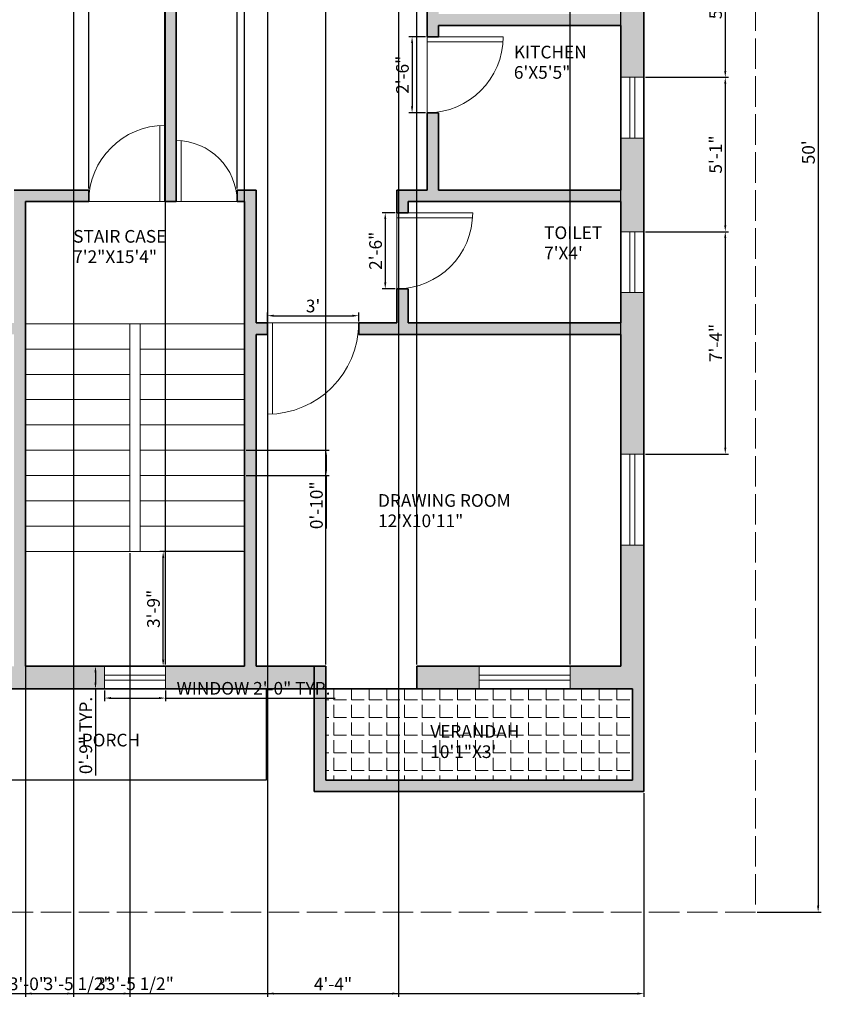
# Model space of a CAD drawing. Units: inches. Extents: x 2871 to 3419, y 1549 to 2228.
# Tile 2 of 3: x 3103 to 3419, y 1549 to 1938. Entities that reach past the tile are written whole.
import ezdxf

# ---------------------------------------------------------------- set-up
doc = ezdxf.new("R2010")
doc.units = ezdxf.units.IN
doc.linetypes.add('ACAD_ISO02W100', pattern=[15, 12, -3])
for name, color, linetype, lineweight in [('A-ANNO-DIMS', 3, 'Continuous', 13), ('A-AREA-IDEN', 3, 'Continuous', 18), ('A-FLOR', 7, 'Continuous', 25), ('A-FLOR-PATT', 30, 'Continuous', 13), ('A-FLOR-STRS', 61, 'Continuous', 18), ('A-WALL-PATT', 18, 'Continuous', 13), ('C-PROP', 7, 'ACAD_ISO02W100', 18), ('doors', 6, 'Continuous', 18), ('wall', 4, 'Continuous', 35), ('windows', 1, 'Continuous', 18)]:
    doc.layers.add(name, color=color, linetype=linetype, lineweight=lineweight)
doc.styles.get("Standard").update_dxf_attribs({"font": 'arial.ttf', "height": 5})
doc.dimstyles.new('ISO-25', dxfattribs={"dimtxt": 5, "dimasz": 2.5, "dimexe": 1.25, "dimexo": 0.625, "dimtad": 1, "dimlunit": 3, "dimtxsty": 'Standard', "dimcen": 2.5, "dimadec": 0, "dimazin": 0, "dimtfac": 1, "dimtmove": 0, "dimatfit": 3, "dimfxl": 1, "dimarcsym": 0})

# ---------------------------------------------------------------- blocks, each defined once
blk = doc.blocks.new('*D6')
at = {"layer": 'A-ANNO-DIMS', "color": 0, "lineweight": -2, "transparency": 16777216}
for p, q in [((3263.29, 1931.24), (3256.74, 1931.24)), ((3257.99, 1928.74), (3257.99, 1903.74)), ((3263.29, 1901.24), (3256.74, 1901.24))]:
    blk.add_line(p, q, dxfattribs=at)
at = {"layer": 'A-ANNO-DIMS', "color": 0, "transparency": 16777216}
for points in [[(3257.58, 1928.74), (3258.41, 1928.74), (3257.99, 1931.24)], [(3257.58, 1903.74), (3258.41, 1903.74), (3257.99, 1901.24)]]:
    blk.add_solid(points, dxfattribs=at)
at = {"layer": 'Defpoints', "color": 0, "transparency": 16777216}
for p in [(3263.92, 1931.24), (3257.99, 1901.24), (3263.92, 1901.24)]:
    blk.add_point(p, dxfattribs=at)
at = {"layer": 'A-ANNO-DIMS', "color": 0, "transparency": 16777216, "insert": (3254.82, 1916.24), "char_height": 5, "attachment_point": 5, "rotation": 90}
blk.add_mtext('2\'-6"', dxfattribs=at)
blk = doc.blocks.new('*D7')
at = {"layer": 'A-ANNO-DIMS', "color": 0, "lineweight": -2, "transparency": 16777216}
for p, q in [((3251.29, 1861.74), (3246.15, 1861.74)), ((3247.4, 1859.24), (3247.4, 1834.24)), ((3251.29, 1831.74), (3246.15, 1831.74))]:
    blk.add_line(p, q, dxfattribs=at)
at = {"layer": 'A-ANNO-DIMS', "color": 0, "transparency": 16777216}
for points in [[(3246.99, 1859.24), (3247.82, 1859.24), (3247.4, 1861.74)], [(3246.99, 1834.24), (3247.82, 1834.24), (3247.4, 1831.74)]]:
    blk.add_solid(points, dxfattribs=at)
at = {"layer": 'Defpoints', "color": 0, "transparency": 16777216}
for p in [(3251.92, 1861.74), (3247.4, 1831.74), (3251.92, 1831.74)]:
    blk.add_point(p, dxfattribs=at)
at = {"layer": 'A-ANNO-DIMS', "color": 0, "transparency": 16777216, "insert": (3244.23, 1846.74), "char_height": 5, "attachment_point": 5, "rotation": 90}
blk.add_mtext('2\'-6"', dxfattribs=at)
blk = doc.blocks.new('*D8')
at = {"layer": 'A-ANNO-DIMS', "color": 0, "lineweight": -2, "transparency": 16777216}
for p, q in [((3200.92, 1818.86), (3200.92, 1822.36)), ((3203.42, 1821.11), (3234.42, 1821.11)), ((3236.92, 1818.86), (3236.92, 1822.36))]:
    blk.add_line(p, q, dxfattribs=at)
at = {"layer": 'A-ANNO-DIMS', "color": 0, "transparency": 16777216}
for points in [[(3203.42, 1821.53), (3203.42, 1820.69), (3200.92, 1821.11)], [(3234.42, 1821.53), (3234.42, 1820.69), (3236.92, 1821.11)]]:
    blk.add_solid(points, dxfattribs=at)
at = {"layer": 'Defpoints', "color": 0, "transparency": 16777216}
for p in [(3236.92, 1821.11), (3200.92, 1818.24), (3236.92, 1818.24)]:
    blk.add_point(p, dxfattribs=at)
at = {"layer": 'A-ANNO-DIMS', "color": 0, "transparency": 16777216, "insert": (3218.92, 1824.29), "char_height": 5, "attachment_point": 5}
blk.add_mtext("3'", dxfattribs=at)
blk = doc.blocks.new('*D13')
at = {"layer": 'A-ANNO-DIMS', "color": 0, "lineweight": -2, "transparency": 16777216}
for p, q in [((3394.09, 2185.62), (3419.45, 2185.62)), ((3418.2, 2183.12), (3418.2, 1588.12)), ((3394.09, 1585.62), (3419.45, 1585.62))]:
    blk.add_line(p, q, dxfattribs=at)
at = {"layer": 'A-ANNO-DIMS', "color": 0, "transparency": 16777216}
for points in [[(3417.79, 2183.12), (3418.62, 2183.12), (3418.2, 2185.62)], [(3417.79, 1588.12), (3418.62, 1588.12), (3418.2, 1585.62)]]:
    blk.add_solid(points, dxfattribs=at)
at = {"layer": 'Defpoints', "color": 0, "transparency": 16777216}
for p in [(3393.47, 2185.62), (3393.47, 1585.62), (3418.2, 1585.62)]:
    blk.add_point(p, dxfattribs=at)
at = {"layer": 'A-ANNO-DIMS', "color": 0, "transparency": 16777216, "insert": (3415.03, 1885.62), "char_height": 5, "attachment_point": 5, "rotation": 90}
blk.add_mtext("50'", dxfattribs=at)
blk = doc.blocks.new('WIN-36IN')
for p, q in [((0, 36), (0, 0)), ((9, 36), (0, 36)), ((3.5, 0), (3.5, 36)), ((5.5, 0), (5.5, 36)), ((9, 0), (9, 36)), ((0, 0), (9, 0))]:
    blk.add_line(p, q)
blk = doc.blocks.new('WIN-24IN')
for p, q in [((0, 24), (0, 0)), ((9, 24), (0, 24)), ((3.5, 0), (3.5, 24)), ((5.5, 0), (5.5, 24)), ((9, 0), (9, 24)), ((0, 0), (9, 0))]:
    blk.add_line(p, q)
blk = doc.blocks.new('DOOR-SWING-30IN')
for p, q in [((28, 29.93), (28, 0)), ((30, 30), (30, 0)), ((30, 0), (0, 0))]:
    blk.add_line(p, q)
blk.add_arc((30, 0), 30, 90, 180)
blk = doc.blocks.new('DOOR-SWING-36IN')
for p, q in [((0, 36), (0, 0)), ((2, 35.94), (2, 0)), ((0, 0), (36, 0))]:
    blk.add_line(p, q)
blk.add_arc((0, 0), 36, 0, 90)
blk = doc.blocks.new('*D20')
at = {"layer": 'A-ANNO-DIMS', "color": 0, "lineweight": -2, "transparency": 16777216}
for p, q in [((3136.67, 1673.11), (3136.67, 1668.89)), ((3160.67, 1673.11), (3160.67, 1668.89)), ((3139.17, 1670.14), (3158.17, 1670.14)), ((3160.67, 1670.14), (3227.69, 1670.14))]:
    blk.add_line(p, q, dxfattribs=at)
at = {"layer": 'A-ANNO-DIMS', "color": 0, "transparency": 16777216}
for points in [[(3139.17, 1670.55), (3139.17, 1669.72), (3136.67, 1670.14)], [(3158.17, 1670.55), (3158.17, 1669.72), (3160.67, 1670.14)]]:
    blk.add_solid(points, dxfattribs=at)
at = {"layer": 'Defpoints', "color": 0, "transparency": 16777216}
for p in [(3136.67, 1673.74), (3160.67, 1673.74), (3160.67, 1670.14)]:
    blk.add_point(p, dxfattribs=at)
at = {"layer": 'A-ANNO-DIMS', "color": 0, "transparency": 16777216, "insert": (3195.43, 1673.35), "char_height": 5, "attachment_point": 5}
blk.add_mtext('WINDOW 2\'-0" TYP.', dxfattribs=at)
blk = doc.blocks.new('*D21')
at = {"layer": 'A-ANNO-DIMS', "color": 0, "lineweight": -2, "transparency": 16777216}
for p, q in [((3136.04, 1682.74), (3131.82, 1682.74)), ((3133.07, 1680.24), (3133.07, 1676.24)), ((3136.04, 1673.74), (3131.82, 1673.74)), ((3133.07, 1673.74), (3133.07, 1639.51))]:
    blk.add_line(p, q, dxfattribs=at)
at = {"layer": 'A-ANNO-DIMS', "color": 0, "transparency": 16777216}
for points in [[(3132.65, 1680.24), (3133.48, 1680.24), (3133.07, 1682.74)], [(3132.65, 1676.24), (3133.48, 1676.24), (3133.07, 1673.74)]]:
    blk.add_solid(points, dxfattribs=at)
at = {"layer": 'Defpoints', "color": 0, "transparency": 16777216}
for p in [(3136.67, 1682.74), (3133.07, 1673.74), (3136.67, 1673.74)]:
    blk.add_point(p, dxfattribs=at)
at = {"layer": 'A-ANNO-DIMS', "color": 0, "transparency": 16777216, "insert": (3129.89, 1655.37), "char_height": 5, "attachment_point": 5, "rotation": 90}
blk.add_mtext('0\'-9" TYP.', dxfattribs=at)
blk = doc.blocks.new('*D22')
at = {"layer": 'A-ANNO-DIMS', "color": 0, "lineweight": -2, "transparency": 16777216}
for p, q in [((2947.92, 1632.61), (2947.92, 1552.22)), ((3349.42, 1632.61), (3349.42, 1552.22)), ((2950.42, 1553.47), (3346.92, 1553.47))]:
    blk.add_line(p, q, dxfattribs=at)
at = {"layer": 'A-ANNO-DIMS', "color": 0, "transparency": 16777216}
for points in [[(2950.42, 1553.89), (2950.42, 1553.05), (2947.92, 1553.47)], [(3346.92, 1553.89), (3346.92, 1553.05), (3349.42, 1553.47)]]:
    blk.add_solid(points, dxfattribs=at)
at = {"layer": 'Defpoints', "color": 0, "transparency": 16777216}
for p in [(2947.92, 1633.24), (3349.42, 1633.24), (3349.42, 1553.47)]:
    blk.add_point(p, dxfattribs=at)
at = {"layer": 'A-ANNO-DIMS', "color": 0, "transparency": 16777216, "insert": (3148.67, 1556.68), "char_height": 5, "attachment_point": 5}
blk.add_mtext('33\'-5 1/2"', dxfattribs=at)
blk = doc.blocks.new('*D27')
at = {"layer": 'A-ANNO-DIMS', "color": 0, "lineweight": -2, "transparency": 16777216}
for p, q in [((3088.42, 2131.11), (3088.42, 1552.22)), ((3124.42, 2131.11), (3124.42, 1552.22)), ((3090.92, 1553.47), (3121.92, 1553.47))]:
    blk.add_line(p, q, dxfattribs=at)
at = {"layer": 'A-ANNO-DIMS', "color": 0, "transparency": 16777216}
for points in [[(3090.92, 1553.89), (3090.92, 1553.05), (3088.42, 1553.47)], [(3121.92, 1553.89), (3121.92, 1553.05), (3124.42, 1553.47)]]:
    blk.add_solid(points, dxfattribs=at)
at = {"layer": 'Defpoints', "color": 0, "transparency": 16777216}
for p in [(3088.42, 2131.74), (3124.42, 2131.74), (3124.42, 1553.47)]:
    blk.add_point(p, dxfattribs=at)
at = {"layer": 'A-ANNO-DIMS', "color": 0, "transparency": 16777216, "insert": (3106.42, 1556.65), "char_height": 5, "attachment_point": 5}
blk.add_mtext('3\'-0"', dxfattribs=at)
blk = doc.blocks.new('*D28')
at = {"layer": 'A-ANNO-DIMS', "color": 0, "lineweight": -2, "transparency": 16777216}
for p, q in [((3200.92, 2131.11), (3200.92, 1552.22)), ((3252.67, 2131.11), (3252.67, 1552.22)), ((3203.42, 1553.47), (3250.17, 1553.47))]:
    blk.add_line(p, q, dxfattribs=at)
at = {"layer": 'A-ANNO-DIMS', "color": 0, "transparency": 16777216}
for points in [[(3203.42, 1553.89), (3203.42, 1553.05), (3200.92, 1553.47)], [(3250.17, 1553.89), (3250.17, 1553.05), (3252.67, 1553.47)]]:
    blk.add_solid(points, dxfattribs=at)
at = {"layer": 'Defpoints', "color": 0, "transparency": 16777216}
for p in [(3200.92, 2131.74), (3252.67, 2131.74), (3252.67, 1553.47)]:
    blk.add_point(p, dxfattribs=at)
at = {"layer": 'A-ANNO-DIMS', "color": 0, "transparency": 16777216, "insert": (3226.79, 1556.6), "char_height": 5, "attachment_point": 5}
blk.add_mtext('4\'-4"', dxfattribs=at)
blk = doc.blocks.new('*D29')
at = {"layer": 'A-ANNO-DIMS', "color": 0, "lineweight": -2, "transparency": 16777216}
for p, q in [((3130.42, 1871.36), (3130.42, 2219.02)), ((3132.92, 2217.77), (3157.92, 2217.77)), ((3160.42, 1871.36), (3160.42, 2219.02))]:
    blk.add_line(p, q, dxfattribs=at)
at = {"layer": 'A-ANNO-DIMS', "color": 0, "transparency": 16777216}
for points in [[(3132.92, 2218.19), (3132.92, 2217.35), (3130.42, 2217.77)], [(3157.92, 2218.19), (3157.92, 2217.35), (3160.42, 2217.77)]]:
    blk.add_solid(points, dxfattribs=at)
at = {"layer": 'Defpoints', "color": 0, "transparency": 16777216}
for p in [(3160.42, 2217.77), (3130.42, 1870.74), (3160.42, 1870.74)]:
    blk.add_point(p, dxfattribs=at)
at = {"layer": 'A-ANNO-DIMS', "color": 0, "transparency": 16777216, "insert": (3145.42, 2220.95), "char_height": 5, "attachment_point": 5}
blk.add_mtext('2\'-6"', dxfattribs=at)
blk = doc.blocks.new('*D30')
at = {"layer": 'A-ANNO-DIMS', "color": 0, "lineweight": -2, "transparency": 16777216}
for p, q in [((3164.92, 1871.36), (3164.92, 2219.02)), ((3167.42, 2217.77), (3186.42, 2217.77)), ((3188.92, 1871.36), (3188.92, 2219.02))]:
    blk.add_line(p, q, dxfattribs=at)
at = {"layer": 'A-ANNO-DIMS', "color": 0, "transparency": 16777216}
for points in [[(3167.42, 2218.19), (3167.42, 2217.35), (3164.92, 2217.77)], [(3186.42, 2218.19), (3186.42, 2217.35), (3188.92, 2217.77)]]:
    blk.add_solid(points, dxfattribs=at)
at = {"layer": 'Defpoints', "color": 0, "transparency": 16777216}
for p in [(3188.92, 2217.77), (3164.92, 1870.74), (3188.92, 1870.74)]:
    blk.add_point(p, dxfattribs=at)
at = {"layer": 'A-ANNO-DIMS', "color": 0, "transparency": 16777216, "insert": (3176.92, 2220.95), "char_height": 5, "attachment_point": 5}
blk.add_mtext('2\'-0"', dxfattribs=at)
blk = doc.blocks.new('*D31')
at = {"layer": 'A-ANNO-DIMS', "color": 0, "lineweight": -2, "transparency": 16777216}
for p, q in [((3191.29, 1727.96), (3158.52, 1727.96)), ((3159.77, 1685.24), (3159.77, 1725.46)), ((3191.29, 1682.74), (3158.52, 1682.74))]:
    blk.add_line(p, q, dxfattribs=at)
at = {"layer": 'A-ANNO-DIMS', "color": 0, "transparency": 16777216}
for points in [[(3159.35, 1725.46), (3160.18, 1725.46), (3159.77, 1727.96)], [(3159.35, 1685.24), (3160.18, 1685.24), (3159.77, 1682.74)]]:
    blk.add_solid(points, dxfattribs=at)
at = {"layer": 'Defpoints', "color": 0, "transparency": 16777216}
for p in [(3159.77, 1727.96), (3191.92, 1727.96), (3191.92, 1682.74)]:
    blk.add_point(p, dxfattribs=at)
at = {"layer": 'A-ANNO-DIMS', "color": 0, "transparency": 16777216, "insert": (3156.59, 1705.35), "char_height": 5, "attachment_point": 5, "rotation": 90}
blk.add_mtext('3\'-9"', dxfattribs=at)
blk = doc.blocks.new('*D32')
at = {"layer": 'A-ANNO-DIMS', "color": 0, "lineweight": -2, "transparency": 16777216}
for p, q in [((3192.54, 1767.96), (3225.32, 1767.96)), ((3224.07, 1765.46), (3224.07, 1760.46)), ((3192.54, 1757.96), (3225.32, 1757.96)), ((3224.07, 1757.96), (3224.07, 1737.03))]:
    blk.add_line(p, q, dxfattribs=at)
at = {"layer": 'A-ANNO-DIMS', "color": 0, "transparency": 16777216}
for points in [[(3223.65, 1765.46), (3224.48, 1765.46), (3224.07, 1767.96)], [(3223.65, 1760.46), (3224.48, 1760.46), (3224.07, 1757.96)]]:
    blk.add_solid(points, dxfattribs=at)
at = {"layer": 'Defpoints', "color": 0, "transparency": 16777216}
for p in [(3191.92, 1767.96), (3191.92, 1757.96), (3224.07, 1757.96)]:
    blk.add_point(p, dxfattribs=at)
at = {"layer": 'A-ANNO-DIMS', "color": 0, "transparency": 16777216, "insert": (3220.89, 1746.25), "char_height": 5, "attachment_point": 5, "rotation": 90}
blk.add_mtext('0\'-10"', dxfattribs=at)
blk = doc.blocks.new('*D33')
at = {"layer": 'A-ANNO-DIMS', "color": 0, "lineweight": -2, "transparency": 16777216}
for p, q in [((3105.42, 1727.34), (3105.42, 1552.22)), ((3146.67, 1727.34), (3146.67, 1552.22)), ((3107.92, 1553.47), (3144.17, 1553.47))]:
    blk.add_line(p, q, dxfattribs=at)
at = {"layer": 'A-ANNO-DIMS', "color": 0, "transparency": 16777216}
for points in [[(3107.92, 1553.89), (3107.92, 1553.05), (3105.42, 1553.47)], [(3144.17, 1553.89), (3144.17, 1553.05), (3146.67, 1553.47)]]:
    blk.add_solid(points, dxfattribs=at)
at = {"layer": 'Defpoints', "color": 0, "transparency": 16777216}
for p in [(3105.42, 1727.96), (3146.67, 1727.96), (3146.67, 1553.47)]:
    blk.add_point(p, dxfattribs=at)
at = {"layer": 'A-ANNO-DIMS', "color": 0, "transparency": 16777216, "insert": (3126.04, 1556.68), "char_height": 5, "attachment_point": 5}
blk.add_mtext('3\'-5 1/2"', dxfattribs=at)
blk = doc.blocks.new('*D36')
at = {"layer": 'A-ANNO-DIMS', "color": 0, "lineweight": -2, "transparency": 16777216}
for p, q in [((3350.04, 1976.24), (3382.82, 1976.24)), ((3381.57, 1973.74), (3381.57, 1917.74)), ((3350.04, 1915.24), (3382.82, 1915.24))]:
    blk.add_line(p, q, dxfattribs=at)
at = {"layer": 'A-ANNO-DIMS', "color": 0, "transparency": 16777216}
for points in [[(3381.15, 1973.74), (3381.98, 1973.74), (3381.57, 1976.24)], [(3381.15, 1917.74), (3381.98, 1917.74), (3381.57, 1915.24)]]:
    blk.add_solid(points, dxfattribs=at)
at = {"layer": 'Defpoints', "color": 0, "transparency": 16777216}
for p in [(3349.42, 1976.24), (3349.42, 1915.24), (3381.57, 1915.24)]:
    blk.add_point(p, dxfattribs=at)
at = {"layer": 'A-ANNO-DIMS', "color": 0, "transparency": 16777216, "insert": (3378.39, 1945.74), "char_height": 5, "attachment_point": 5, "rotation": 90}
blk.add_mtext('5\'-1"', dxfattribs=at)
blk = doc.blocks.new('*D37')
at = {"layer": 'A-ANNO-DIMS', "color": 0, "lineweight": -2, "transparency": 16777216}
for p, q in [((3350.04, 1915.24), (3382.82, 1915.24)), ((3381.57, 1912.74), (3381.57, 1856.74)), ((3350.04, 1854.24), (3382.82, 1854.24))]:
    blk.add_line(p, q, dxfattribs=at)
at = {"layer": 'A-ANNO-DIMS', "color": 0, "transparency": 16777216}
for points in [[(3381.15, 1912.74), (3381.98, 1912.74), (3381.57, 1915.24)], [(3381.15, 1856.74), (3381.98, 1856.74), (3381.57, 1854.24)]]:
    blk.add_solid(points, dxfattribs=at)
at = {"layer": 'Defpoints', "color": 0, "transparency": 16777216}
for p in [(3349.42, 1915.24), (3349.42, 1854.24), (3381.57, 1854.24)]:
    blk.add_point(p, dxfattribs=at)
at = {"layer": 'A-ANNO-DIMS', "color": 0, "transparency": 16777216, "insert": (3378.39, 1884.74), "char_height": 5, "attachment_point": 5, "rotation": 90}
blk.add_mtext('5\'-1"', dxfattribs=at)
blk = doc.blocks.new('*D38')
at = {"layer": 'A-ANNO-DIMS', "color": 0, "lineweight": -2, "transparency": 16777216}
for p, q in [((3350.04, 1854.24), (3382.82, 1854.24)), ((3381.57, 1851.74), (3381.57, 1768.95)), ((3350.04, 1766.45), (3382.82, 1766.45))]:
    blk.add_line(p, q, dxfattribs=at)
at = {"layer": 'A-ANNO-DIMS', "color": 0, "transparency": 16777216}
for points in [[(3381.15, 1851.74), (3381.98, 1851.74), (3381.57, 1854.24)], [(3381.15, 1768.95), (3381.98, 1768.95), (3381.57, 1766.45)]]:
    blk.add_solid(points, dxfattribs=at)
at = {"layer": 'Defpoints', "color": 0, "transparency": 16777216}
for p in [(3349.42, 1854.24), (3349.42, 1766.45), (3381.57, 1766.45)]:
    blk.add_point(p, dxfattribs=at)
at = {"layer": 'A-ANNO-DIMS', "color": 0, "transparency": 16777216, "insert": (3378.44, 1810.34), "char_height": 5, "attachment_point": 5, "rotation": 90}
blk.add_mtext('7\'-4"', dxfattribs=at)
blk = doc.blocks.new('*D45')
at = {"layer": 'A-ANNO-DIMS', "color": 0, "lineweight": -2, "transparency": 16777216}
for p, q in [((3320.42, 1683.36), (3320.42, 2219.02)), ((3322.92, 2217.77), (3337.92, 2217.77)), ((3340.42, 1683.36), (3340.42, 2219.02))]:
    blk.add_line(p, q, dxfattribs=at)
at = {"layer": 'A-ANNO-DIMS', "color": 0, "transparency": 16777216}
for points in [[(3322.92, 2218.19), (3322.92, 2217.35), (3320.42, 2217.77)], [(3337.92, 2218.19), (3337.92, 2217.35), (3340.42, 2217.77)]]:
    blk.add_solid(points, dxfattribs=at)
at = {"layer": 'Defpoints', "color": 0, "transparency": 16777216}
for p in [(3340.42, 2217.77), (3320.42, 1682.74), (3340.42, 1682.74)]:
    blk.add_point(p, dxfattribs=at)
at = {"layer": 'A-ANNO-DIMS', "color": 0, "transparency": 16777216, "insert": (3330.42, 2220.95), "char_height": 5, "attachment_point": 5}
blk.add_mtext('1\'-8"', dxfattribs=at)
blk = doc.blocks.new('*D47')
at = {"layer": 'A-ANNO-DIMS', "color": 0, "lineweight": -2, "transparency": 16777216}
for p, q in [((3223.92, 1683.36), (3223.92, 2219.02)), ((3226.42, 2217.77), (3257.42, 2217.77)), ((3259.92, 1683.36), (3259.92, 2219.02))]:
    blk.add_line(p, q, dxfattribs=at)
at = {"layer": 'A-ANNO-DIMS', "color": 0, "transparency": 16777216}
for points in [[(3226.42, 2218.19), (3226.42, 2217.35), (3223.92, 2217.77)], [(3257.42, 2218.19), (3257.42, 2217.35), (3259.92, 2217.77)]]:
    blk.add_solid(points, dxfattribs=at)
at = {"layer": 'Defpoints', "color": 0, "transparency": 16777216}
for p in [(3259.92, 2217.77), (3223.92, 1682.74), (3259.92, 1682.74)]:
    blk.add_point(p, dxfattribs=at)
at = {"layer": 'A-ANNO-DIMS', "color": 0, "transparency": 16777216, "insert": (3241.92, 2220.95), "char_height": 5, "attachment_point": 5}
blk.add_mtext('3\'-0"', dxfattribs=at)
blk = doc.blocks.new('*D49')
at = {"layer": 'A-ANNO-DIMS', "color": 0, "lineweight": -2, "transparency": 16777216}
for p, q in [((3259.92, 1683.36), (3259.92, 2219.02)), ((3262.42, 2217.77), (3317.92, 2217.77)), ((3320.42, 1683.36), (3320.42, 2219.02))]:
    blk.add_line(p, q, dxfattribs=at)
at = {"layer": 'A-ANNO-DIMS', "color": 0, "transparency": 16777216}
for points in [[(3262.42, 2218.19), (3262.42, 2217.35), (3259.92, 2217.77)], [(3317.92, 2218.19), (3317.92, 2217.35), (3320.42, 2217.77)]]:
    blk.add_solid(points, dxfattribs=at)
at = {"layer": 'Defpoints', "color": 0, "transparency": 16777216}
for p in [(3320.42, 2217.77), (3259.92, 1682.74), (3320.42, 1682.74)]:
    blk.add_point(p, dxfattribs=at)
at = {"layer": 'A-ANNO-DIMS', "color": 0, "transparency": 16777216, "insert": (3290.17, 2220.98), "char_height": 5, "attachment_point": 5}
blk.add_mtext('5\'-0 1/2"', dxfattribs=at)
blk = doc.blocks.new('*D51')
at = {"layer": 'A-ANNO-DIMS', "color": 0, "lineweight": -2, "transparency": 16777216}
for p, q in [((3160.67, 1683.36), (3160.67, 2219.02)), ((3163.17, 2217.77), (3189.42, 2217.77)), ((3191.92, 1683.36), (3191.92, 2219.02))]:
    blk.add_line(p, q, dxfattribs=at)
at = {"layer": 'A-ANNO-DIMS', "color": 0, "transparency": 16777216}
for points in [[(3163.17, 2218.19), (3163.17, 2217.35), (3160.67, 2217.77)], [(3189.42, 2218.19), (3189.42, 2217.35), (3191.92, 2217.77)]]:
    blk.add_solid(points, dxfattribs=at)
at = {"layer": 'Defpoints', "color": 0, "transparency": 16777216}
for p in [(3191.92, 2217.77), (3160.67, 1682.74), (3191.92, 1682.74)]:
    blk.add_point(p, dxfattribs=at)
at = {"layer": 'A-ANNO-DIMS', "color": 0, "transparency": 16777216, "insert": (3176.29, 2220.98), "char_height": 5, "attachment_point": 5}
blk.add_mtext('2\'-7 1/2"', dxfattribs=at)

msp = doc.modelspace()

# ---------------------------------------------------------------- hatches: boundary and pattern name
at = {"layer": 'A-FLOR-PATT'}
h = msp.add_hatch(dxfattribs=at)
h.set_pattern_fill('ANGLE', color=256)
h.set_pattern_definition([(0, (0, 0), (0, 6.985), [5.08, -1.905]), (90, (0, 0), (-6.985, 4e-16), [5.08, -1.905])])
h.paths.add_polyline_path([(3073.418, 1673.735), (3037.418, 1673.735), (2952.418, 1673.735), (2952.418, 1637.735), (3073.418, 1637.735)])
h.paths.add_polyline_path([(3344.918, 1673.735), (3259.918, 1673.735), (3223.918, 1673.735), (3223.918, 1637.735), (3344.918, 1637.735)])
h.paths.add_polyline_path([(2998.155, 1645.095), (3026.055, 1645.095), (3026.055, 1652.758), (2998.155, 1652.758)], flags=24)
h.paths.add_polyline_path([(2998.183, 1653.243), (3039.496, 1653.243), (3039.496, 1660.743), (2998.183, 1660.743)], flags=24)
h.paths.add_polyline_path([(3263.884, 1645.095), (3291.783, 1645.095), (3291.783, 1652.758), (3263.884, 1652.758)], flags=24)
h.paths.add_polyline_path([(3263.911, 1653.243), (3305.224, 1653.243), (3305.224, 1660.743), (3263.911, 1660.743)], flags=24)
at = {"layer": 'A-WALL-PATT'}
h = msp.add_hatch(color=256, dxfattribs=at)
h.dxf.hatch_style = 1
h.paths.add_polyline_path([(2956.918, 2131.735), (3002.418, 2131.735), (3002.418, 2140.735), (2947.918, 2140.735), (2947.918, 2079.154), (2956.918, 2079.154)])
h.paths.add_polyline_path([(3252.668, 2140.735), (3160.418, 2140.735), (3160.418, 2131.735), (3196.418, 2131.735), (3196.418, 1992.735), (3128.918, 1992.735), (3128.918, 1988.235), (3160.418, 1988.235), (3160.418, 1870.735), (3160.418, 1866.235), (3164.918, 1866.235), (3164.918, 1890.235), (3164.918, 1988.235), (3205.418, 1988.235), (3205.418, 1992.735), (3200.918, 1992.735), (3200.918, 2131.735), (3252.668, 2131.735)])
h.paths.add_polyline_path([(3349.418, 2140.735), (3288.668, 2140.735), (3288.668, 2131.735), (3340.418, 2131.735), (3340.418, 2080.235), (3349.418, 2080.235)])
h.paths.add_polyline_path([(3349.418, 2044.235), (3340.418, 2044.235), (3340.418, 1992.735), (3302.918, 1992.735), (3302.918, 1988.235), (3340.418, 1988.235), (3340.418, 1976.235), (3349.418, 1976.235)])
h.paths.add_polyline_path([(3349.418, 1952.235), (3340.418, 1952.235), (3340.418, 1940.235), (3268.418, 1940.235), (3268.418, 1988.235), (3272.918, 1988.235), (3272.918, 1992.735), (3241.418, 1992.735), (3241.418, 1988.235), (3263.918, 1988.235), (3263.918, 1931.235), (3268.418, 1931.235), (3268.418, 1935.735), (3340.418, 1935.735), (3340.418, 1915.235), (3349.418, 1915.235)])
h.paths.add_polyline_path([(3349.418, 1891.235), (3340.418, 1891.235), (3340.418, 1870.735), (3268.418, 1870.735), (3268.418, 1901.235), (3263.918, 1901.235), (3263.918, 1870.735), (3251.918, 1870.735), (3251.918, 1866.235), (3251.918, 1861.735), (3256.418, 1861.735), (3256.418, 1866.235), (3340.418, 1866.235), (3340.418, 1854.235), (3349.418, 1854.235)])
h.paths.add_polyline_path([(3349.418, 1830.235), (3340.418, 1830.235), (3340.418, 1818.235), (3256.418, 1818.235), (3256.418, 1831.735), (3251.918, 1831.735), (3251.918, 1818.235), (3236.918, 1818.235), (3236.918, 1813.735), (3340.418, 1813.735), (3340.418, 1766.452), (3349.418, 1766.452)])
h.paths.add_polyline_path([(3349.418, 1730.452), (3340.418, 1730.452), (3340.418, 1682.735), (3320.418, 1682.735), (3320.418, 1673.735), (3344.918, 1673.735), (3344.918, 1637.735), (3223.918, 1637.735), (3223.918, 1673.735), (3219.418, 1673.735), (3219.418, 1633.235), (3349.418, 1633.235)])
h.paths.add_polyline_path([(3284.418, 1682.735), (3259.918, 1682.735), (3259.918, 1673.735), (3284.418, 1673.735)], flags=17)
h.paths.add_polyline_path([(3223.918, 1682.735), (3219.418, 1682.735), (3219.418, 1673.735), (3223.918, 1673.735)], flags=17)
h.paths.add_polyline_path([(3196.418, 1813.735), (3200.918, 1813.735), (3200.918, 1818.235), (3196.418, 1818.235), (3196.418, 1866.235), (3196.418, 1870.735), (3188.918, 1870.735), (3188.918, 1866.235), (3191.918, 1866.235), (3191.918, 1682.735), (3160.668, 1682.735), (3160.668, 1673.735), (3219.418, 1673.735), (3219.418, 1682.735), (3196.418, 1682.735)])
h.paths.add_polyline_path([(3105.418, 1866.235), (3130.418, 1866.235), (3130.418, 1870.735), (3100.918, 1870.735), (3100.918, 1866.235), (3100.918, 1818.235), (3096.418, 1818.235), (3096.418, 1813.735), (3100.918, 1813.735), (3100.918, 1682.735), (3077.918, 1682.735), (3077.918, 1673.735), (3136.668, 1673.735), (3136.668, 1682.735), (3105.418, 1682.735)])
h.paths.add_polyline_path([(3077.918, 1682.735), (3073.418, 1682.735), (3073.418, 1673.735), (3077.918, 1673.735)], flags=17)
h.paths.add_polyline_path([(3077.918, 1673.735), (3073.418, 1673.735), (3073.418, 1637.735), (2952.418, 1637.735), (2952.418, 1673.735), (2976.918, 1673.735), (2976.918, 1682.735), (2956.918, 1682.735), (2956.918, 1729.593), (2947.918, 1729.593), (2947.918, 1633.235), (3077.918, 1633.235)])
h.paths.add_polyline_path([(3037.418, 1682.735), (3012.918, 1682.735), (3012.918, 1673.735), (3037.418, 1673.735)], flags=17)
h.paths.add_polyline_path([(3060.418, 1818.235), (3045.418, 1818.235), (3045.418, 1831.735), (3040.918, 1831.735), (3040.918, 1818.235), (2956.918, 1818.235), (2956.918, 1830.772), (2947.918, 1830.772), (2947.918, 1765.593), (2956.918, 1765.593), (2956.918, 1813.735), (3060.418, 1813.735)])
h.paths.add_polyline_path([(3045.418, 1870.735), (3033.418, 1870.735), (3033.418, 1901.235), (3028.918, 1901.235), (3028.918, 1870.735), (2956.918, 1870.735), (2956.918, 1891.289), (2947.918, 1891.289), (2947.918, 1854.772), (2956.918, 1854.772), (2956.918, 1866.235), (3040.918, 1866.235), (3040.918, 1861.735), (3045.418, 1861.735), (3045.418, 1866.235)])
h.paths.add_polyline_path([(3033.418, 1988.235), (3043.418, 1988.235), (3043.418, 1992.735), (3024.418, 1992.735), (3024.418, 1988.235), (3028.918, 1988.235), (3028.918, 1940.235), (2956.918, 1940.235), (2956.918, 1952.063), (2947.918, 1952.063), (2947.918, 1915.289), (2956.918, 1915.289), (2956.918, 1935.735), (3028.918, 1935.735), (3028.918, 1931.235), (3033.418, 1931.235)])
h.paths.add_polyline_path([(2956.918, 2043.154), (2947.918, 2043.154), (2947.918, 1976.063), (2956.918, 1976.063), (2956.918, 1988.235), (2994.418, 1988.235), (2994.418, 1992.735), (2956.918, 1992.735)])

# ---------------------------------------------------------------- linework, layer by layer
at = {"layer": 'A-FLOR'}
for p, q in [((3200.352, 1673.735), (3200.352, 1637.735)), ((3200.352, 1637.735), (3097.318, 1637.735))]:
    msp.add_line(p, q, dxfattribs=at)
at = {"layer": 'A-FLOR-STRS'}
for p, q in [((3191.918, 1817.96), (3105.418, 1817.96)), ((3146.668, 1817.96), (3146.668, 1727.96)), ((3150.668, 1817.96), (3150.668, 1727.96)), ((3146.668, 1807.96), (3105.418, 1807.96)), ((3191.918, 1807.96), (3150.668, 1807.96)), ((3146.668, 1797.96), (3105.418, 1797.96)), ((3191.918, 1797.96), (3150.668, 1797.96)), ((3146.668, 1787.96), (3105.418, 1787.96)), ((3191.918, 1787.96), (3150.668, 1787.96)), ((3146.668, 1777.96), (3105.418, 1777.96)), ((3191.918, 1777.96), (3150.668, 1777.96)), ((3146.668, 1767.96), (3105.418, 1767.96)), ((3191.918, 1767.96), (3150.668, 1767.96)), ((3146.668, 1757.96), (3105.418, 1757.96)), ((3191.918, 1757.96), (3150.668, 1757.96)), ((3146.668, 1747.96), (3105.418, 1747.96)), ((3191.918, 1747.96), (3150.668, 1747.96)), ((3146.668, 1737.96), (3105.418, 1737.96)), ((3191.918, 1737.96), (3150.668, 1737.96)), ((3191.918, 1727.96), (3105.418, 1727.96))]:
    msp.add_line(p, q, dxfattribs=at)
at = {"layer": 'C-PROP'}
for p, q in [((3393.468, 2185.622), (3393.468, 1585.622)), ((3393.468, 1585.622), (2913.468, 1585.622))]:
    msp.add_line(p, q, dxfattribs=at)
at = {"layer": 'doors'}
for p, q in [((3164.918, 1890.235), (3164.918, 1866.235)), ((3166.918, 1890.152), (3166.918, 1866.235)), ((3164.918, 1866.235), (3188.918, 1866.235))]:
    msp.add_line(p, q, dxfattribs=at)
msp.add_arc((3164.918, 1866.235), 24, 0, 90, dxfattribs=at)
at = {"layer": 'wall'}
for p, q in [((3349.418, 2140.735), (3349.418, 1633.235)), ((3160.418, 1988.235), (3160.418, 1870.735)), ((3164.918, 1988.235), (3164.918, 1870.735)), ((3263.918, 1988.235), (3263.918, 1931.235)), ((3340.418, 1935.735), (3268.418, 1935.735)), ((3268.418, 1935.735), (3268.418, 1931.235)), ((3340.418, 1935.735), (3340.418, 1870.735)), ((3268.418, 1931.235), (3263.918, 1931.235)), ((3268.418, 1901.235), (3263.918, 1901.235)), ((3263.918, 1901.235), (3263.918, 1870.735)), ((3268.418, 1901.235), (3268.418, 1870.735)), ((3130.418, 1870.735), (3100.918, 1870.735)), ((3130.418, 1870.735), (3130.418, 1866.235)), ((3160.418, 1870.735), (3160.418, 1866.235)), ((3164.918, 1870.735), (3164.918, 1866.235)), ((3188.918, 1870.735), (3188.918, 1866.235)), ((3196.418, 1870.735), (3188.918, 1870.735)), ((3196.418, 1866.235), (3196.418, 1870.735)), ((3263.918, 1870.735), (3251.918, 1870.735)), ((3251.918, 1866.235), (3251.918, 1870.735)), ((3340.418, 1870.735), (3268.418, 1870.735)), ((3105.418, 1866.235), (3105.418, 1682.735)), ((3130.418, 1866.235), (3105.418, 1866.235)), ((3164.918, 1866.235), (3160.418, 1866.235)), ((3191.918, 1866.235), (3188.918, 1866.235)), ((3191.918, 1866.235), (3191.918, 1682.735)), ((3196.418, 1866.235), (3196.418, 1818.235)), ((3251.918, 1866.235), (3251.918, 1861.735)), ((3340.418, 1866.235), (3256.418, 1866.235)), ((3256.418, 1866.235), (3256.418, 1861.735)), ((3340.418, 1866.235), (3340.418, 1818.235)), ((3256.418, 1861.735), (3251.918, 1861.735)), ((3256.418, 1831.735), (3251.918, 1831.735)), ((3251.918, 1831.735), (3251.918, 1818.235)), ((3256.418, 1831.735), (3256.418, 1818.235)), ((3200.918, 1818.235), (3196.418, 1818.235)), ((3200.918, 1818.235), (3200.918, 1813.735)), ((3236.918, 1818.235), (3236.918, 1813.735)), ((3251.918, 1818.235), (3236.918, 1818.235)), ((3340.418, 1818.235), (3256.418, 1818.235)), ((3200.918, 1813.735), (3196.418, 1813.735)), ((3196.418, 1813.735), (3196.418, 1682.735)), ((3340.418, 1813.735), (3236.918, 1813.735)), ((3340.418, 1813.735), (3340.418, 1682.735)), ((3191.918, 1682.735), (3105.418, 1682.735)), ((3223.918, 1682.735), (3196.418, 1682.735)), ((3219.418, 1682.735), (3219.418, 1633.235)), ((3223.918, 1673.735), (3223.918, 1682.735)), ((3340.418, 1682.735), (3259.918, 1682.735)), ((3259.918, 1673.735), (3259.918, 1682.735)), ((3223.918, 1673.735), (3073.418, 1673.735)), ((3223.918, 1673.735), (3223.918, 1637.735)), ((3223.918, 1673.735), (3259.918, 1673.735)), ((3344.918, 1673.735), (3259.918, 1673.735)), ((3344.918, 1673.735), (3344.918, 1637.735)), ((3344.918, 1637.735), (3223.918, 1637.735)), ((3349.418, 1633.235), (3219.418, 1633.235))]:
    msp.add_line(p, q, dxfattribs=at)

# ---------------------------------------------------------------- block references
at = {"layer": 'doors', "extrusion": (0, 0, -1), "zscale": -1}
for name, p, rotation in [('DOOR-SWING-30IN', (-3263.918, 1901.235), 89.99999999999882), ('DOOR-SWING-30IN', (-3251.918, 1831.735), 89.99999999999882), ('DOOR-SWING-36IN', (-3200.918, 1818.235), 180)]:
    msp.add_blockref(name, p, dxfattribs=dict(at, rotation=rotation))
at = {"layer": 'doors'}
msp.add_blockref('DOOR-SWING-30IN', (3130.418, 1866.235), dxfattribs=at)
at = {"layer": 'windows'}
for p in [(3340.418, 1891.235), (3340.418, 1830.235)]:
    msp.add_blockref('WIN-24IN', p, dxfattribs=at)
for name, p, rotation in [('WIN-36IN', (3349.419, 1766.452), 180), ('WIN-24IN', (3136.668, 1682.735), 270.0000000000003), ('WIN-36IN', (3284.418, 1682.735), 269.999999999999)]:
    msp.add_blockref(name, p, dxfattribs=dict(at, rotation=rotation))

# ---------------------------------------------------------------- texts
at = {"layer": 'A-AREA-IDEN'}
for s, p in [('KITCHEN', (3298.151, 1922.702)), ('6\'X5\'5"', (3298.151, 1914.67)), ('STAIR CASE', (3124.269, 1849.945)), ('TOILET', (3310.082, 1851.375)), ('7\'2"X15\'4"', (3124.269, 1841.913)), ("7'X4'", (3310.082, 1843.343)), ('DRAWING ROOM', (3244.558, 1745.654)), ('12\'X10\'11"', (3244.558, 1737.622)), ('PORCH', (3127.625, 1651.051)), ('VERANDAH', (3265.161, 1654.493)), ('10\'1"X3\'', (3265.161, 1646.461))]:
    msp.add_text(s, height=5, dxfattribs=at).set_placement(p)

# ---------------------------------------------------------------- dimensions: what is measured, and where the dimension line sits
at = {"layer": 'A-ANNO-DIMS'}
for base, p1, p2, override, picture, middle in [((3191.918308, 2217.771512), (3160.668308, 1682.735115), (3191.918308, 1682.735115), {"dimdec": 1, "dimlfac": 1, "dimrnd": 0, "dimzin": 1, "dimdsep": 46, "dimlunit": 4, "dimfrac": 2}, '*D51', (3176.293308, 2220.98177803)), ((3320.418, 2217.772), (3259.918, 1682.735), (3320.418, 1682.735), {"dimdec": 1, "dimlfac": 1, "dimrnd": 0, "dimzin": 1, "dimdsep": 46, "dimlunit": 4, "dimfrac": 2}, '*D49', (3290.168, 2220.982)), ((3160.418, 2217.772), (3130.418, 1870.735), (3160.418, 1870.735), {"dimdec": 1, "dimlfac": 1, "dimrnd": 0, "dimzin": 1, "dimdsep": 46, "dimlunit": 4, "dimfrac": 2}, '*D29', (3145.418, 2220.949)), ((3188.918, 2217.772), (3164.918, 1870.735), (3188.918, 1870.735), {"dimdec": 1, "dimlfac": 1, "dimrnd": 0, "dimzin": 1, "dimdsep": 46, "dimlunit": 4, "dimfrac": 2}, '*D30', (3176.918, 2220.949)), ((3259.918, 2217.772), (3223.918, 1682.735), (3259.918, 1682.735), {"dimdec": 1, "dimlfac": 1, "dimrnd": 0, "dimzin": 1, "dimdsep": 46, "dimlunit": 4, "dimfrac": 2}, '*D47', (3241.918, 2220.951)), ((3340.418, 2217.772), (3320.418, 1682.735), (3340.418, 1682.735), {"dimdec": 1, "dimlfac": 1, "dimrnd": 0, "dimzin": 1, "dimdsep": 46, "dimlunit": 4, "dimfrac": 2}, '*D45', (3330.418, 2220.949)), ((3124.418, 1553.472), (3088.418, 2131.735), (3124.418, 2131.735), {"dimdec": 1, "dimlfac": 1, "dimrnd": 0, "dimzin": 1, "dimdsep": 46, "dimlunit": 4, "dimfrac": 2}, '*D27', (3106.418, 1556.651)), ((3252.668308, 1553.471512), (3200.918308, 2131.735115), (3252.668308, 2131.735115), {"dimdec": 1, "dimlfac": 1, "dimrnd": 0, "dimzin": 1, "dimdsep": 46, "dimlunit": 4, "dimfrac": 2}, '*D28', (3226.793308, 1556.596512)), ((3236.918, 1821.111), (3200.918, 1818.235), (3236.918, 1818.235), {"dimclrd": 0, "dimclre": 0, "dimclrt": 0}, '*D8', (3218.918, 1824.29)), ((3146.668308, 1553.471512), (3105.418308, 1727.960327), (3146.668308, 1727.960327), {"dimdec": 1, "dimlfac": 1, "dimrnd": 0, "dimzin": 1, "dimdsep": 46, "dimlunit": 4, "dimfrac": 2}, '*D33', (3126.043308, 1556.683483351)), ((3349.418, 1553.472), (2947.918, 1633.235), (3349.418, 1633.235), {"dimdec": 1, "dimlfac": 1, "dimrnd": 0, "dimzin": 1, "dimdsep": 46, "dimlunit": 4, "dimfrac": 2}, '*D22', (3148.668, 1556.683))]:
    dim = msp.add_linear_dim(base=base, p1=p1, p2=p2, dimstyle='ISO-25', override=override, dxfattribs=at)
    dim.commit()
    dim.dimension.update_dxf_attribs({"geometry": picture, "text_midpoint": middle})
for base, p1, p2, angle, override, picture, middle in [((3418.204, 1585.622), (3393.468, 2185.622), (3393.468, 1585.622), 90, {"dimclrd": 0, "dimclre": 0, "dimclrt": 0}, '*D13', (3415.026, 1885.622)), ((3381.568, 1915.235), (3349.418, 1976.235), (3349.418, 1915.235), 270, {"dimdec": 1, "dimlfac": 1, "dimrnd": 0, "dimzin": 1, "dimdsep": 46, "dimlunit": 4, "dimfrac": 2}, '*D36', (3378.39, 1945.735)), ((3257.995, 1901.235), (3263.918, 1931.235), (3263.918, 1901.235), 90, {"dimclrd": 0, "dimclre": 0, "dimclrt": 0}, '*D6', (3254.817, 1916.235)), ((3381.568, 1854.235), (3349.418, 1915.235), (3349.418, 1854.235), 270, {"dimdec": 1, "dimlfac": 1, "dimrnd": 0, "dimzin": 1, "dimdsep": 46, "dimlunit": 4, "dimfrac": 2}, '*D37', (3378.39, 1884.735)), ((3247.405, 1831.735), (3251.918, 1861.735), (3251.918, 1831.735), 90, {"dimclrd": 0, "dimclre": 0, "dimclrt": 0}, '*D7', (3244.227, 1846.735)), ((3381.568, 1766.452), (3349.418, 1854.235), (3349.418, 1766.452), 270, {"dimdec": 1, "dimlfac": 1, "dimrnd": 0, "dimzin": 1, "dimdsep": 46, "dimlunit": 4, "dimfrac": 2}, '*D38', (3378.443, 1810.344)), ((3224.068, 1757.96), (3191.918, 1767.96), (3191.918, 1757.96), 270, {"dimdec": 1, "dimlfac": 1, "dimrnd": 0, "dimzin": 1, "dimdsep": 46, "dimlunit": 4, "dimfrac": 2}, '*D32', (3220.89, 1746.247)), ((3159.768, 1727.96), (3191.918, 1682.735), (3191.918, 1727.96), 90, {"dimdec": 1, "dimlfac": 1, "dimrnd": 0, "dimzin": 1, "dimdsep": 46, "dimlunit": 4, "dimfrac": 2}, '*D31', (3156.589, 1705.348))]:
    dim = msp.add_linear_dim(base=base, p1=p1, p2=p2, angle=angle, dimstyle='ISO-25', override=override, dxfattribs=at)
    dim.commit()
    dim.dimension.update_dxf_attribs({"geometry": picture, "text_midpoint": middle})
for base, p1, p2, angle, text, picture, middle in [((3160.668, 1670.135), (3136.668, 1673.735), (3160.668, 1673.735), 0, 'WINDOW <> TYP.', '*D20', (3195.429, 1673.347)), ((3133.068, 1673.735), (3136.668, 1682.735), (3136.668, 1673.735), 270, '<> TYP.', '*D21', (3129.89, 1655.371))]:
    dim = msp.add_linear_dim(base=base, p1=p1, p2=p2, angle=angle, text=text, dimstyle='ISO-25', override={"dimdec": 1, "dimlfac": 1, "dimrnd": 0, "dimzin": 1, "dimdsep": 46, "dimlunit": 4, "dimfrac": 2}, dxfattribs=at)
    dim.commit()
    dim.dimension.update_dxf_attribs({"geometry": picture, "text_midpoint": middle})

doc.saveas('drawing.dxf')
